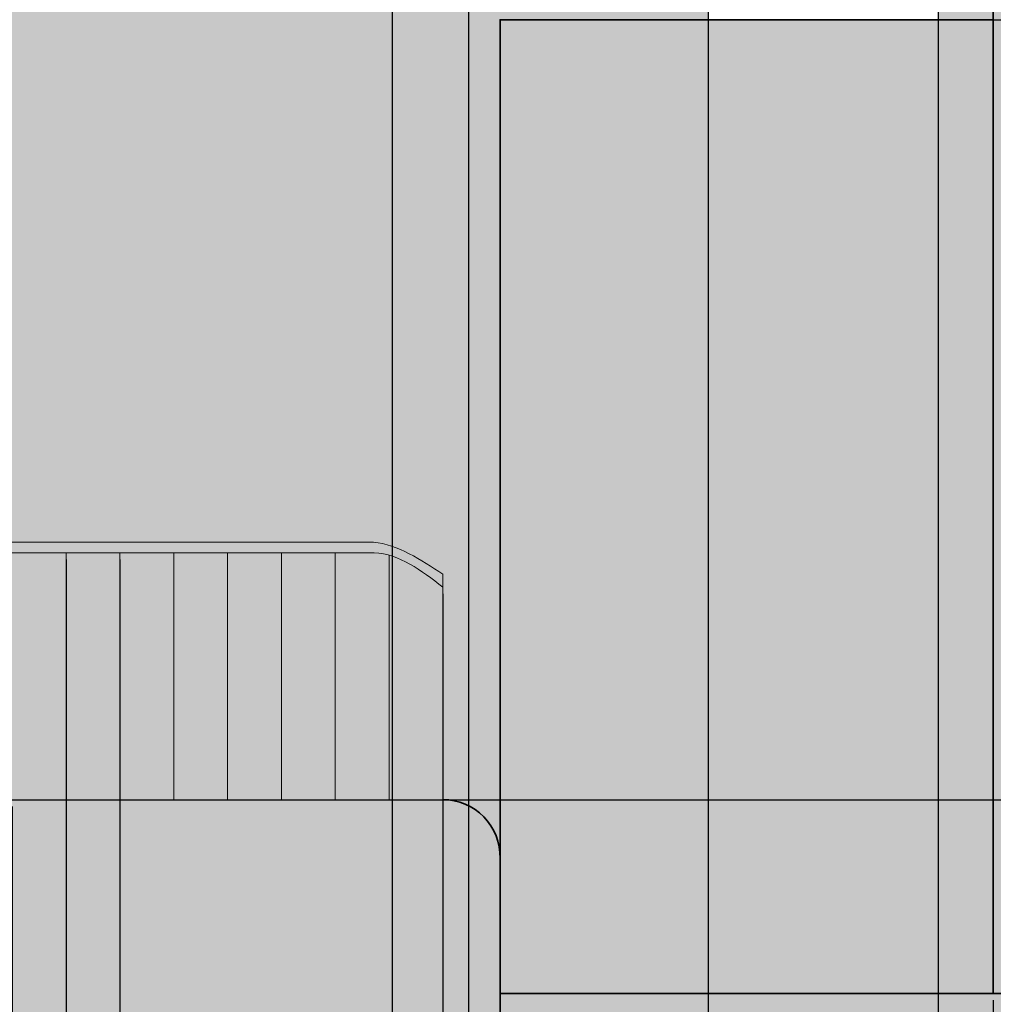
# Model space of a CAD drawing. Units: inches. Extents: x 18 to 59.8, y 2.7 to 81.2.
# Tile 6 of 9: x 44.4 to 53.4, y 29.5 to 38.7. Entities that reach past the tile are written whole.
import ezdxf

# ---------------------------------------------------------------- set-up
doc = ezdxf.new("R2010")
doc.units = ezdxf.units.IN
doc.header["$MEASUREMENT"] = 0
for name, color, linetype, lineweight in [('A-ANNO-DIMS', 2, 'Continuous', 18), ('A-ELEV', 7, 'Continuous', 35), ('A-ELEV-PATT', 8, 'Continuous', 13), ('A-ELEV-RAIL', 7, 'Continuous', 18)]:
    doc.layers.add(name, color=color, linetype=linetype, lineweight=lineweight)
doc.styles.get("Standard").update_dxf_attribs({"font": 'arial.ttf'})
doc.dimstyles.get("Standard").update_dxf_attribs({"dimtxt": 0.18, "dimasz": 0.18, "dimexe": 0.18, "dimexo": 0.0625, "dimgap": 0.09, "dimtad": 0, "dimtih": 1, "dimtoh": 1, "dimdec": 1, "dimzin": 0, "dimdsep": 46, "dimlunit": 3, "dimtxsty": 'Standard', "dimcen": 0.09, "dimadec": 0, "dimazin": 0, "dimtfac": 1, "dimtdec": 1, "dimtofl": 0, "dimtmove": 0, "dimatfit": 3, "dimfxl": 1, "dimtolj": 1, "dimtzin": 0, "dimarcsym": 0})

# ---------------------------------------------------------------- blocks, each defined once
blk = doc.blocks.new('*D23')
at = {"layer": 'A-ANNO-DIMS', "color": 0, "lineweight": -2, "transparency": 16777216}
for p, q in [((48.859971, 29.578248), (48.859971, 2.670747999999999)), ((53.440061, 29.578248), (53.440061, 2.670747999999999)), ((49.039971, 2.850747999999999), (50.82243073396998, 2.850747999999999)), ((53.260061, 2.850747999999999), (51.47760126603001, 2.850747999999999))]:
    blk.add_line(p, q, dxfattribs=at)
at = {"layer": 'A-ANNO-DIMS', "color": 0, "transparency": 16777216}
for points in [[(49.039971, 2.880747999999999), (49.039971, 2.820748), (48.859971, 2.850747999999999)], [(53.260061, 2.880747999999999), (53.260061, 2.820748), (53.440061, 2.850747999999999)]]:
    blk.add_solid(points, dxfattribs=at)
at = {"layer": 'Defpoints', "color": 0, "transparency": 16777216}
for p in [(48.859971, 29.640748), (53.440061, 29.640748), (53.440061, 2.850747999999999)]:
    blk.add_point(p, dxfattribs=at)
at = {"layer": 'A-ANNO-DIMS', "color": 0, "transparency": 16777216, "insert": (51.150016, 2.850747999999999), "char_height": 0.18, "attachment_point": 5}
blk.add_mtext('\\A1;4.58', dxfattribs=at)
blk = doc.blocks.new('*D24')
at = {"layer": 'A-ANNO-DIMS', "color": 0, "lineweight": -2, "transparency": 16777216}
for p, q in [((48.859971, 38.622063), (48.859971, 2.670748000000003)), ((50.792976, 38.622063), (50.792976, 2.670748000000003)), ((49.039971, 2.850747999999999), (49.44124157639837, 2.850747999999999)), ((50.612976, 2.850747999999999), (50.21170542360164, 2.850747999999999))]:
    blk.add_line(p, q, dxfattribs=at)
at = {"layer": 'A-ANNO-DIMS', "color": 0, "transparency": 16777216}
for points in [[(49.039971, 2.880747999999999), (49.039971, 2.820748), (48.859971, 2.850747999999999)], [(50.612976, 2.880747999999999), (50.612976, 2.820748), (50.792976, 2.850747999999999)]]:
    blk.add_solid(points, dxfattribs=at)
at = {"layer": 'Defpoints', "color": 0, "transparency": 16777216}
for p in [(48.859971, 38.684563), (50.792976, 38.684563), (50.792976, 2.850747999999999)]:
    blk.add_point(p, dxfattribs=at)
at = {"layer": 'A-ANNO-DIMS', "color": 0, "transparency": 16777216, "insert": (49.8264735, 2.850747999999999), "char_height": 0.18, "attachment_point": 5}
blk.add_mtext('\\A1;1.933', dxfattribs=at)
blk = doc.blocks.new('*D25')
at = {"layer": 'A-ANNO-DIMS', "color": 0, "lineweight": -2, "transparency": 16777216}
for p, q in [((50.792976, 41.253458), (50.792976, 2.670748000000003)), ((52.926966, 41.253458), (52.926966, 2.670748000000003)), ((50.972976, 2.850747999999999), (51.46510060436562, 2.850747999999999)), ((52.746966, 2.850747999999999), (52.25484139563437, 2.850747999999999))]:
    blk.add_line(p, q, dxfattribs=at)
at = {"layer": 'A-ANNO-DIMS', "color": 0, "transparency": 16777216}
for points in [[(50.972976, 2.880747999999999), (50.972976, 2.820748), (50.792976, 2.850747999999999)], [(52.746966, 2.880747999999999), (52.746966, 2.820748), (52.926966, 2.850747999999999)]]:
    blk.add_solid(points, dxfattribs=at)
at = {"layer": 'Defpoints', "color": 0, "transparency": 16777216}
for p in [(50.792976, 41.315958), (52.926966, 41.315958), (52.926966, 2.850747999999999)]:
    blk.add_point(p, dxfattribs=at)
at = {"layer": 'A-ANNO-DIMS', "color": 0, "transparency": 16777216, "insert": (51.859971, 2.850747999999999), "char_height": 0.18, "attachment_point": 5}
blk.add_mtext('\\A1;2.134', dxfattribs=at)
blk = doc.blocks.new('*D26')
at = {"layer": 'A-ANNO-DIMS', "color": 0, "lineweight": -2, "transparency": 16777216}
for p, q in [((52.98946600000003, 41.31595800000002), (59.62997100000006, 41.31595800000002)), ((59.44997100000005, 41.13595800000001), (59.44997100000005, 40.18222502933153)), ((59.44997100000005, 38.86456300000001), (59.44997100000005, 39.8182959706685)), ((52.98946600000003, 38.68456300000001), (59.62997100000006, 38.68456300000001))]:
    blk.add_line(p, q, dxfattribs=at)
at = {"layer": 'A-ANNO-DIMS', "color": 0, "transparency": 16777216}
for points in [[(59.41997100000005, 41.13595800000001), (59.47997100000005, 41.13595800000001), (59.44997100000005, 41.31595800000002)], [(59.41997100000005, 38.86456300000001), (59.47997100000005, 38.86456300000001), (59.44997100000005, 38.68456300000001)]]:
    blk.add_solid(points, dxfattribs=at)
at = {"layer": 'Defpoints', "color": 0, "transparency": 16777216}
for p in [(52.92696600000002, 41.31595800000002), (59.44997100000005, 41.31595800000002), (52.92696600000002, 38.68456300000001)]:
    blk.add_point(p, dxfattribs=at)
at = {"layer": 'A-ANNO-DIMS', "color": 0, "transparency": 16777216, "insert": (59.44997100000005, 40.00026049999998), "char_height": 0.18, "attachment_point": 5}
blk.add_mtext('\\A1;2.63', dxfattribs=at)
blk = doc.blocks.new('*D27')
at = {"layer": 'A-ANNO-DIMS', "color": 0, "lineweight": -2, "transparency": 16777216}
for p, q in [((30.46859000000001, 31.44074800000002), (59.62997100000006, 31.44074800000002)), ((59.44997100000005, 31.26074800000002), (59.44997100000005, 30.72265113778992)), ((59.44997100000005, 29.82074800000002), (59.44997100000005, 30.35884486221011)), ((48.92247100000003, 29.64074800000001), (59.62997100000006, 29.64074800000002))]:
    blk.add_line(p, q, dxfattribs=at)
at = {"layer": 'A-ANNO-DIMS', "color": 0, "transparency": 16777216}
for points in [[(59.41997100000005, 31.26074800000002), (59.47997100000005, 31.26074800000002), (59.44997100000005, 31.44074800000002)], [(59.41997100000005, 29.82074800000002), (59.47997100000005, 29.82074800000002), (59.44997100000005, 29.64074800000002)]]:
    blk.add_solid(points, dxfattribs=at)
at = {"layer": 'Defpoints', "color": 0, "transparency": 16777216}
for p in [(30.40609000000002, 31.44074800000002), (48.85997100000003, 29.64074800000001), (59.44997100000005, 29.64074800000002)]:
    blk.add_point(p, dxfattribs=at)
at = {"layer": 'A-ANNO-DIMS', "color": 0, "transparency": 16777216, "insert": (59.44997100000005, 30.54074799999999), "char_height": 0.18, "attachment_point": 5}
blk.add_mtext('\\A1;1.8', dxfattribs=at)
blk = doc.blocks.new('*D54')
at = {"layer": 'A-ANNO-DIMS', "color": 0, "lineweight": -2, "transparency": 16777216}
for p, q in [((28.258258, 33.771141), (28.258258, 2.670747999999999)), ((48.330239, 33.351579), (48.330239, 2.670747999999999)), ((28.438258, 2.850747999999999), (37.89900975511596, 2.850747999999999)), ((48.15023899999999, 2.850747999999999), (38.68948724488403, 2.850747999999999))]:
    blk.add_line(p, q, dxfattribs=at)
at = {"layer": 'A-ANNO-DIMS', "color": 0, "transparency": 16777216}
for points in [[(28.438258, 2.880747999999999), (28.438258, 2.820748), (28.258258, 2.850747999999999)], [(48.15023899999999, 2.880747999999999), (48.15023899999999, 2.820748), (48.330239, 2.850747999999999)]]:
    blk.add_solid(points, dxfattribs=at)
at = {"layer": 'Defpoints', "color": 0, "transparency": 16777216}
for p in [(28.258258, 33.833641), (48.330239, 33.414079), (48.330239, 2.850747999999999)]:
    blk.add_point(p, dxfattribs=at)
at = {"layer": 'A-ANNO-DIMS', "color": 0, "transparency": 16777216, "insert": (38.2942485, 2.850747999999999), "char_height": 0.18, "attachment_point": 5}
blk.add_mtext('\\A1;20.07', dxfattribs=at)
blk = doc.blocks.new('*D55')
at = {"layer": 'A-ANNO-DIMS', "color": 0, "lineweight": -2, "transparency": 16777216}
for p, q in [((44.830239, 33.671141), (44.830239, 2.670747999999999)), ((45.33023899999999, 33.671141), (45.33023899999999, 2.670747999999999)), ((44.650239, 2.850747999999999), (44.470239, 2.850747999999999)), ((45.51023899999999, 2.850747999999999), (45.690239, 2.850747999999999))]:
    blk.add_line(p, q, dxfattribs=at)
at = {"layer": 'A-ANNO-DIMS', "color": 0, "transparency": 16777216}
for points in [[(44.650239, 2.880747999999999), (44.650239, 2.820748), (44.830239, 2.850747999999999)], [(45.51023899999999, 2.880747999999999), (45.51023899999999, 2.820748), (45.33023899999999, 2.850747999999999)]]:
    blk.add_solid(points, dxfattribs=at)
at = {"layer": 'Defpoints', "color": 0, "transparency": 16777216}
for p in [(44.830239, 33.733641), (45.33023899999999, 33.733641), (45.33023899999999, 2.850747999999999)]:
    blk.add_point(p, dxfattribs=at)
at = {"layer": 'A-ANNO-DIMS', "color": 0, "transparency": 16777216, "insert": (45.94476833151432, 2.850747999999999), "char_height": 0.18, "attachment_point": 5}
blk.add_mtext('\\A1;0.5', dxfattribs=at)
blk = doc.blocks.new('*D58')
at = {"layer": 'A-ANNO-DIMS', "color": 0, "lineweight": -2, "transparency": 16777216}
for p, q in [((48.859971, 38.622063), (48.859971, 2.670748000000003)), ((44.330239, 31.378248), (44.330239, 2.670747999999999)), ((44.510239, 2.850747999999999), (46.26770390859482, 2.850747999999999)), ((48.679971, 2.850747999999999), (46.92250609140518, 2.850747999999999))]:
    blk.add_line(p, q, dxfattribs=at)
at = {"layer": 'A-ANNO-DIMS', "color": 0, "transparency": 16777216}
for points in [[(44.510239, 2.880747999999999), (44.510239, 2.820748), (44.330239, 2.850747999999999)], [(48.679971, 2.880747999999999), (48.679971, 2.820748), (48.859971, 2.850747999999999)]]:
    blk.add_solid(points, dxfattribs=at)
at = {"layer": 'Defpoints', "color": 0, "transparency": 16777216}
for p in [(48.859971, 38.684563), (44.330239, 31.440748), (48.859971, 2.850747999999999)]:
    blk.add_point(p, dxfattribs=at)
at = {"layer": 'A-ANNO-DIMS', "color": 0, "transparency": 16777216, "insert": (46.595105, 2.850747999999999), "char_height": 0.18, "attachment_point": 5}
blk.add_mtext('\\A1;4.53', dxfattribs=at)
blk = doc.blocks.new('*D61')
at = {"layer": 'A-ANNO-DIMS', "color": 0, "lineweight": -2, "transparency": 16777216}
for p, q in [((32.233824, 49.378248), (32.233824, 2.670748000000003)), ((47.859971, 49.378248), (47.859971, 2.670748000000003)), ((32.413824, 2.850747999999999), (39.59180200204638, 2.850747999999999)), ((47.679971, 2.850747999999999), (40.50199299795361, 2.850747999999999))]:
    blk.add_line(p, q, dxfattribs=at)
at = {"layer": 'A-ANNO-DIMS', "color": 0, "transparency": 16777216}
for points in [[(32.413824, 2.880747999999999), (32.413824, 2.820748), (32.233824, 2.850747999999999)], [(47.679971, 2.880747999999999), (47.679971, 2.820748), (47.859971, 2.850747999999999)]]:
    blk.add_solid(points, dxfattribs=at)
at = {"layer": 'Defpoints', "color": 0, "transparency": 16777216}
for p in [(32.233824, 49.440748), (47.859971, 49.440748), (47.859971, 2.850747999999999)]:
    blk.add_point(p, dxfattribs=at)
at = {"layer": 'A-ANNO-DIMS', "color": 0, "transparency": 16777216, "insert": (40.04689749999999, 2.850747999999999), "char_height": 0.18, "attachment_point": 5}
blk.add_mtext('\\A1;15.626', dxfattribs=at)
blk = doc.blocks.new('*D66')
at = {"layer": 'A-ANNO-DIMS', "color": 0, "lineweight": -2, "transparency": 16777216}
for p, q in [((28.803543, 51.378248), (28.803543, 2.670748000000003)), ((48.567078, 51.179103), (48.567078, 2.670748000000003)), ((28.983543, 2.850747999999999), (38.23052195975444, 2.850747999999999)), ((48.387078, 2.850747999999999), (39.14009904024556, 2.850747999999999))]:
    blk.add_line(p, q, dxfattribs=at)
at = {"layer": 'A-ANNO-DIMS', "color": 0, "transparency": 16777216}
for points in [[(28.983543, 2.880747999999999), (28.983543, 2.820748), (28.803543, 2.850747999999999)], [(48.387078, 2.880747999999999), (48.387078, 2.820748), (48.567078, 2.850747999999999)]]:
    blk.add_solid(points, dxfattribs=at)
at = {"layer": 'Defpoints', "color": 0, "transparency": 16777216}
for p in [(28.803543, 51.440748), (48.567078, 51.24160299999999), (48.567078, 2.850747999999999)]:
    blk.add_point(p, dxfattribs=at)
at = {"layer": 'A-ANNO-DIMS', "color": 0, "transparency": 16777216, "insert": (38.6853105, 2.850747999999999), "char_height": 0.18, "attachment_point": 5}
blk.add_mtext('\\A1;19.764', dxfattribs=at)

msp = doc.modelspace()

# ---------------------------------------------------------------- hatches: boundary and pattern name
at = {"layer": 'A-ELEV-PATT'}
h = msp.add_hatch(color=256, dxfattribs=at)
h.set_gradient(color1=(255, 255, 255), color2=(199, 200, 202))
h.paths.add_polyline_path([(38.85997087182833, 75.45212783007513, 0.4125526599533602), (36.85997087192615, 77.44074750583997), (21.85997087182832, 77.44074750583995), (21.85997087182832, 22.44074750583995), (22.85997087182833, 22.44074750583995), (48.85997087182833, 22.44074750583996), (48.85997087182833, 30.92342676155402, 0.4074472928332927), (48.33023903111634, 31.44074750583995), (30.40609029701442, 31.44074750583996, -0.7603989452129261), (34.01164157247843, 44.44074750583996), (47.85997087182832, 44.44074750583995, -0.4142135623730951), (48.85997087182833, 43.44074750583994), (48.85997087182833, 48.44074750583995, 0.4142135623730955), (47.85997087182832, 49.44074750583995), (32.23382408177119, 49.44074750583993, -0.2243141867862321), (27.84111392101349, 52.84266085519661, -0.8480128940945467), (38.85997087182833, 61.44074750583993)])
h.paths.add_polyline_path([(55.85997087182832, 77.44074750583995), (54.85997087182832, 77.44074750583997), (54.85997087182832, 22.24074750583996), (55.85997087182832, 22.24074750583995)])
h.paths.add_polyline_path([(54.85997087182832, 51.54074750583995), (53.44006084017791, 51.54074750583996), (53.44006084017792, 29.64074750583996), (54.85997087182832, 29.64074750583996)])
h.paths.add_polyline_path([(54.85997087182832, 61.44074750583993), (53.44006084017791, 57.44074750583993), (53.44006084017791, 51.64074750583996), (54.85997087182832, 51.64074750583996)])
h.paths.add_polyline_path([(54.85997087182832, 29.44074750583995), (54.47100875861361, 29.44074750583995), (54.47100875861361, 22.24074750583996), (54.85997087182832, 22.24074750583996)])
h.paths.add_polyline_path([(55.57447446325177, 22.24074750583995), (54.85997087182832, 22.24074750583996), (54.57447446325178, 22.24074750583996), (53.93466996146642, 21.792542566958), (54.58769880335594, 21.54947740208223)])
h.paths.add_polyline_path([(54.59913950424823, 21.54521903603421), (53.94430429933965, 21.78895655088426), (53.94430429933965, 18.44074750583995), (54.59913950424823, 18.44074750583995)])
h.paths.add_polyline_path([(53.94430429933965, 21.78895655088427), (53.93466996146642, 21.792542566958), (53.58162006229036, 21.54521903603422), (53.58162006229036, 18.44074750583995), (53.94430429933965, 18.44074750583994)])
h.paths.add_polyline_path([(53.36475139777029, 20.69276091189374), (52.89555240690669, 21.06460517556268), (52.89555240690669, 18.44074750583995), (53.3647513977703, 18.44074750583994)])
h.paths.add_polyline_path([(52.89555240690669, 21.06460517556268), (50.57752474318004, 19.44074750583995), (50.57752474318004, 18.44074750583995), (52.89555240690669, 18.44074750583995)])
h.paths.add_polyline_path([(53.58162006229036, 21.54521903603423), (52.89555240690668, 21.06460517556268), (53.3647513977703, 20.69276091189373), (53.58162006229036, 20.84468482967704)])
h.paths.add_polyline_path([(26.81093959479239, 19.44074750583995), (24.96715419074249, 20.84074750583995), (24.96715419074249, 18.44074750583995), (26.81093959479239, 18.44074750583995)])
h.paths.add_polyline_path([(24.96715419074249, 20.84074750583995), (24.41645576890079, 20.84268308307895), (24.41645576890079, 18.44074750583994), (24.96715419074249, 18.44074750583994)])
h.paths.add_polyline_path([(24.41645576890079, 20.84268308307895), (24.41645576890079, 21.25889692219009), (24.05877847081848, 21.5304839605815), (24.03006070560372, 21.51834150822755), (24.03006070560372, 18.44074750583995), (24.41645576890079, 18.44074750583995)])
h.paths.add_polyline_path([(24.03006070560372, 21.51834150822755), (23.41645576890078, 21.2588969221901), (23.41645576890078, 18.44074750583996), (24.03006070560372, 18.44074750583995)])
h.paths.add_polyline_path([(24.03006070560372, 21.51834150822755), (24.05877847081849, 21.53048396058151), (23.12336878669258, 22.24074750583995), (22.12336878669259, 22.24074750583996), (23.41645576890079, 21.2588969221901)])
h.paths.add_polyline_path([(24.41645576890079, 21.2588969221901), (24.41645576890079, 20.84268308307896), (24.96715419074249, 20.84074750583994)])
h.paths.add_polyline_path([(47.85997087182832, 18.44074750583995), (29.85997087182832, 18.44074750583995), (29.85997087182832, 6.440747505839951), (30.85997087182832, 6.440747505839937), (30.85997087182832, 17.44074750583995), (38.85997087182833, 17.44074750583995), (46.85997087182832, 17.44074750583995), (46.85997087182832, 6.440747505839937), (47.85997087182832, 6.440747505839958)])
h.paths.add_polyline_path([(54.57559250001032, 15.2149800477124), (54.57559250001032, 6.440747505839944), (55.85997087182832, 6.440747505839951), (55.85997087182832, 18.44074750583995), (47.85997087182832, 18.44074750583995), (47.85997087182832, 6.440747505839944), (49.14824210254597, 6.440747505839944), (49.14824210254597, 15.2149800477124, -1)])
h = msp.add_hatch(dxfattribs=at)
h.set_pattern_fill('ANSI31', color=256, scale=5, angle=45, style=0)
h.set_pattern_definition([(90, (0, 0), (-0.6250000000000001, 0), [])])
h.paths.add_polyline_path([(54.85997087182832, 69.44074750583995), (38.85997087182833, 69.44074750583995), (38.85997087182833, 61.44074750583995), (54.85997087182832, 61.44074750583994)])
h.paths.add_polyline_path([(54.85997087182833, 61.44074750583994), (38.85997087182833, 61.44074750583995), (36.85997087182832, 61.44074750583993, 0.4434140223301819), (27.69861713021859, 58.44074750583995), (48.85997087182833, 58.44074750583995), (48.85997087182833, 57.44074750583994), (53.44006084017792, 57.44074750583995)])
h.paths.add_polyline_path([(37.16613704638868, 59.85769359025997), (37.11866134610267, 59.85769359025997), (37.11866134610267, 59.93991004599954), (37.49943513222304, 59.93991004599954), (37.49943513222304, 59.85769359025997), (37.45195943193702, 59.85769359025997, -3.476462016968403)], flags=16)
h.paths.add_polyline_path([(42.66000754223224, 59.8390978600294), (42.61253184194623, 59.8390978600294), (42.61253184194623, 59.92131431576897), (42.9933056280666, 59.92131431576897), (42.9933056280666, 59.8390978600294), (42.94582992778058, 59.8390978600294, -3.47646201696846)], flags=16)
h.paths.add_polyline_path([(49.64399186138049, 60.00882068949565), (49.59651616109447, 60.00882068949565), (49.59651616109447, 60.09103714523522), (49.97728994721485, 60.09103714523522), (49.97728994721485, 60.00882068949565), (49.92981424692883, 60.00882068949565, -3.476462016968434)], flags=16)
h.paths.add_polyline_path([(44.46707765301489, 57.04074750583994), (32.6670776530149, 57.04074750583994), (32.6670776530149, 56.04074750583993), (44.46707765301489, 56.04074750583993)])
h.paths.add_polyline_path([(47.85997087182831, 43.44074750583994), (46.85997087182832, 43.44074750583994), (34.0116415724774, 43.44074750583994, 0.2012982920418866), (29.34810857035394, 41.44074750583995), (47.85997087182831, 41.44074750583995, 1)])
h.paths.add_polyline_path([(36.60163289663952, 42.55241488062237), (36.55415719635351, 42.55241488062236), (36.55415719635351, 42.63463133636193), (36.93493098247388, 42.63463133636193), (36.93493098247388, 42.55241488062236), (36.88745528218787, 42.55241488062236, -3.476462016968307)], flags=16)
h.paths.add_polyline_path([(42.98647563665846, 42.5780367704526), (42.93899993637245, 42.5780367704526), (42.93899993637245, 42.66025322619216), (43.31977372249282, 42.66025322619216), (43.31977372249282, 42.57803677045259), (43.2722980222068, 42.57803677045259, -3.476462016968351)], flags=16)
h.paths.add_polyline_path([(54.47100875861361, 29.44074750583995), (48.85997087182833, 29.44074750583995), (48.85997087182833, 22.24074750583995), (54.47100875861361, 22.24074750583994)])
h.paths.add_polyline_path([(54.57447446325179, 22.24074750583995), (23.12336878669258, 22.24074750583995), (26.81093959479238, 19.44074750583996), (50.57752474318005, 19.44074750583996)])
h.paths.add_polyline_path([(54.57559250001032, 15.2149800477124, 1), (49.14824210254597, 15.2149800477124), (49.14824210254597, 6.440747505839958), (54.57559250001032, 6.440747505839944)])
h.paths.add_polyline_path([(49.83226884926398, 9.122455521673542), (49.66565363924473, 9.122455521673537), (49.66565363924473, 12.60204276083839), (49.83226884926398, 12.6020427608384)], flags=16)
at = {"layer": 'A-ELEV-PATT', "transparency": 33554620}
h = msp.add_hatch(color=256, dxfattribs=at)
h.set_gradient(color1=(147, 149, 152))
edge = h.paths.add_edge_path()
edge.add_line((32.5670776530149, 55.94074750583994), (32.5670776530149, 57.14074750583994))
edge.add_line((32.5670776530149, 57.14074750583994), (44.5670776530149, 57.14074750583994))
edge.add_line((44.5670776530149, 57.14074750583994), (44.5670776530149, 55.94074750583994))
edge.add_line((44.5670776530149, 55.94074750583994), (44.56707765301487, 51.54074750583998))
edge.add_line((44.56707765301487, 51.54074750583998), (47.92075940082271, 51.54074750583998))
edge.add_spline(control_points=[(47.92075940082271, 51.54074750583998), (48.15238228194087, 51.51452682454292), (48.35972996747788, 51.37806491819363), (48.56707765301488, 51.24160301184435)], knot_values=[0, 0, 0, 0, 0.7121900809507601, 0.7121900809507601, 0.7121900809507601, 0.7121900809507601], degree=3, periodic=0)
edge.add_line((48.56707765301488, 51.24160301184435), (48.56707765301488, 49.14785428702649))
edge.add_arc((47.85997087182832, 48.44074750583995), 1, 5.739170477267294, 44.999999999999375, ccw=False)
edge.add_line((48.85495830893494, 48.54074750583996), (48.85997087182833, 48.54074750583996))
edge.add_line((48.85997087182833, 48.54074750583996), (48.85997087182833, 49.44074750583995))
edge.add_line((48.85997087182833, 49.44074750583995), (48.85997087182833, 58.44074750583995))
edge.add_line((48.85997087182833, 58.44074750583995), (27.6986171302186, 58.44074750583995))
edge.add_arc((33.63815495998532, 55.79107886226907), 6.503756879831279, 155.9580213816849, 220.80747886606)
edge.add_line((28.71539791616241, 51.54074750583994), (32.5670776530149, 51.54074750583994))
edge.add_line((32.5670776530149, 51.54074750583994), (32.5670776530149, 55.94074750583994))
edge = h.paths.add_edge_path()
edge.add_line((32.33023903111487, 40.44074750583996), (35.33023903111486, 40.44074750583996))
edge.add_line((35.33023903111486, 40.44074750583996), (38.33023903111485, 40.44074750583996))
edge.add_line((38.33023903111485, 40.44074750583996), (41.33023903111483, 40.44074750583996))
edge.add_line((41.33023903111483, 40.44074750583996), (44.33023903111482, 40.44074750583996))
edge.add_line((44.33023903111482, 40.44074750583996), (44.33023903111482, 33.83364072465343))
edge.add_line((44.33023903111482, 33.83364072465343), (47.68392077892264, 33.83364072465344))
edge.add_spline(control_points=[(47.68392077892267, 33.83364072465344), (47.91554366004082, 33.80742004335637), (48.12289134557783, 33.67095813700708), (48.33023903111483, 33.5344962306578)], knot_values=[0, 0, 0, 0, 0.7121900809507601, 0.7121900809507601, 0.7121900809507601, 0.7121900809507601], degree=3, periodic=0)
edge.add_line((48.33023903111483, 33.5344962306578), (48.33023903111483, 31.44074750583995))
edge.add_arc((48.3303844405005, 30.91101568508362), 0.5297318407134953, 1.3425044870115812, 90.01572747485528, ccw=False)
edge.add_line((48.85997087182833, 30.92342676155392), (48.85997087182833, 38.68456317332766))
edge.add_line((48.85997087182833, 38.68456317332766), (50.79297551695841, 38.68456317332766))
edge.add_line((50.79297551695841, 38.68456317332766), (50.79297551695841, 41.31595823441438))
edge.add_line((50.79297551695841, 41.31595823441438), (52.92696622669824, 41.31595823441438))
edge.add_line((52.92696622669824, 41.31595823441438), (52.92696622669824, 38.68456317332766))
edge.add_line((52.92696622669824, 38.68456317332766), (53.44006084017791, 38.68456317332766))
edge.add_line((53.44006084017791, 38.68456317332766), (53.44006084017791, 48.44074750583995))
edge.add_line((53.44006084017791, 48.44074750583995), (48.85997087182833, 48.44074750583995))
edge.add_line((48.85997087182833, 48.44074750583995), (48.85997087182832, 42.44074750583995))
edge.add_arc((47.85997087182831, 42.44074750583995), 1, -90, 0, ccw=False)
edge.add_line((47.85997087182831, 41.44074750583995), (29.34810857035394, 41.44074750583995))
edge.add_arc((34.06310194306089, 36.8836189221075), 6.557330511217327, 135.9754091201121, 207.7183105881144)
edge.add_line((28.25825772220566, 33.83364072465339), (32.33023903111487, 33.83364072465341))
edge.add_line((32.33023903111487, 33.83364072465341), (32.33023903111487, 40.44074750583996))
h.paths.add_polyline_path([(53.44006084017791, 57.44074750583995), (48.85997087182833, 57.44074750583994), (48.85997087182833, 51.64074750583996), (53.44006084017791, 51.64074750583996)])
h.paths.add_polyline_path([(29.56707765301488, 51.44074750583992), (28.80354322363853, 51.44074750583992, 0.040450980236505), (29.56707765301488, 50.71907894974708)], flags=17)
h.paths.add_polyline_path([(30.06707765301488, 51.44074750583992), (29.56707765301488, 51.44074750583992), (29.56707765301488, 50.71907894974708, 0.0237787432624053), (30.06707765301488, 50.35543166808938)], flags=17)
h.paths.add_polyline_path([(30.56707765301487, 51.44074750583993), (30.06707765301488, 51.44074750583992), (30.06707765301488, 50.35543166808938, 0.0223728768734236), (30.56707765301488, 50.05807461261393)], flags=17)
h.paths.add_polyline_path([(31.06707765301487, 51.44074750583993), (30.56707765301487, 51.44074750583993), (30.56707765301488, 50.05807461261393, 0.021345047641792), (31.06707765301488, 49.8171007041625)], flags=17)
h.paths.add_polyline_path([(31.56707765301487, 51.44074750583993), (31.06707765301487, 51.44074750583993), (31.06707765301488, 49.8171007041625, 0.0205857748313696), (31.56707765301488, 49.62589497689267)], flags=17)
h.paths.add_polyline_path([(32.06707765301488, 51.44074750583993), (31.56707765301487, 51.44074750583993), (31.56707765301488, 49.62589497689267, 0.0200299041308402), (32.06707765301488, 49.47993240164282)], flags=17)
h.paths.add_polyline_path([(32.5670776530149, 51.44074750583993), (32.06707765301488, 51.44074750583993), (32.06707765301488, 49.47993240164282, 0.0065845078177353), (32.23382408177119, 49.44074750583993), (32.5670776530149, 49.44074750583993)], flags=17)
h.paths.add_polyline_path([(45.06707765301486, 51.44074750583996), (44.56707765301487, 51.44074750583996), (44.56707765301487, 49.44074750583995), (45.06707765301488, 49.44074750583995)], flags=17)
h.paths.add_polyline_path([(45.56707765301488, 51.44074750583996), (45.06707765301486, 51.44074750583996), (45.06707765301488, 49.44074750583995), (45.56707765301488, 49.44074750583995)], flags=17)
h.paths.add_polyline_path([(46.06707765301488, 51.44074750583996), (45.56707765301488, 51.44074750583996), (45.56707765301488, 49.44074750583995), (46.06707765301488, 49.44074750583995)], flags=17)
h.paths.add_polyline_path([(46.56707765301487, 51.44074750583996), (46.06707765301488, 51.44074750583996), (46.06707765301488, 49.44074750583995), (46.56707765301487, 49.44074750583995)], flags=17)
h.paths.add_polyline_path([(47.06707765301487, 51.44074750583996), (46.56707765301487, 51.44074750583996), (46.56707765301487, 49.44074750583995), (47.06707765301487, 49.44074750583995)], flags=17)
h.paths.add_polyline_path([(47.56707765301487, 51.44074750583996), (47.06707765301487, 51.44074750583996), (47.06707765301487, 49.44074750583995), (47.56707765301488, 49.44074750583995)], flags=17)
edge = h.paths.add_edge_path(flags=17)
edge.add_spline(control_points=[(48.06707765301273, 51.41840713962396), (48.02172392661717, 51.43105064440995), (47.97524027779975, 51.4389035969284), (47.92733930740307, 51.44074750583996)], knot_values=[0.5701039528936005, 0.5701039528936005, 0.5701039528936005, 0.5701039528936005, 0.7151116034373463, 0.7151116034373463, 0.7151116034373463, 0.7151116034373644], degree=3, periodic=0)
edge.add_line((47.92733930740307, 51.44074750583996), (47.56707765301487, 51.44074750583996))
edge.add_line((47.56707765301487, 51.44074750583996), (47.56707765301488, 49.44074750583995))
edge.add_line((47.56707765301488, 49.44074750583995), (47.85997087182832, 49.44074750583995))
edge.add_arc((47.85997087182832, 48.44074750583995), 1, 78.04714410929728, 90, ccw=False)
edge.add_line((48.06707765301489, 49.41906584931846), (48.06707765301488, 51.41840713962341))
edge = h.paths.add_edge_path(flags=17)
edge.add_spline(control_points=[(48.56707765301488, 51.12118615879595), (48.40623273758901, 51.24494240176197), (48.24538782216315, 51.36869864472799), (48.06707765301273, 51.41840713962396)], knot_values=[0, 0, 0, 0, 0.5701039528936005, 0.5701039528936005, 0.5701039528936005, 0.5701039528936005], degree=3, periodic=0)
edge.add_line((48.06707765301488, 51.41840713962327), (48.06707765301489, 49.41906584931846))
edge.add_arc((47.85997087182832, 48.44074750583995), 1, 44.999999999999375, 78.04714410929728, ccw=False)
edge.add_line((48.56707765301488, 49.14785428702649), (48.56707765301488, 51.12118615879595))
h.paths.add_polyline_path([(49.35997087182833, 51.54074750583996), (48.85997087182833, 51.54074750583996), (48.85997087182833, 49.44074750583995), (48.85997087182833, 48.54074750583996), (49.35997087182833, 48.54074750583996)])
h.paths.add_polyline_path([(49.85997087182834, 51.54074750583996), (49.35997087182833, 51.54074750583996), (49.35997087182833, 48.54074750583996), (49.85997087182833, 48.54074750583996)])
h.paths.add_polyline_path([(50.35997087182834, 51.54074750583996), (49.85997087182834, 51.54074750583996), (49.85997087182833, 48.54074750583996), (50.35997087182833, 48.54074750583996)])
h.paths.add_polyline_path([(50.85997087182834, 51.54074750583996), (50.35997087182834, 51.54074750583996), (50.35997087182832, 48.54074750583996), (50.85997087182833, 48.54074750583996)])
h.paths.add_polyline_path([(51.35997087182833, 51.54074750583996), (50.85997087182834, 51.54074750583996), (50.85997087182833, 48.54074750583996), (51.35997087182833, 48.54074750583996)])
h.paths.add_polyline_path([(51.85997087182833, 51.54074750583996), (51.35997087182833, 51.54074750583996), (51.35997087182833, 48.54074750583995), (51.85997087182832, 48.54074750583995)])
h.paths.add_polyline_path([(52.35997087182834, 51.54074750583995), (51.85997087182833, 51.54074750583996), (51.85997087182832, 48.54074750583995), (52.35997087182834, 48.54074750583995)])
h.paths.add_polyline_path([(52.85997087182835, 51.54074750583995), (52.35997087182834, 51.54074750583995), (52.35997087182834, 48.54074750583995), (52.85997087182833, 48.54074750583995)])
h.paths.add_polyline_path([(53.35997087182834, 51.54074750583995), (52.85997087182835, 51.54074750583995), (52.85997087182833, 48.54074750583995), (53.35997087182834, 48.54074750583995)])
h.paths.add_polyline_path([(53.44006084017792, 38.68456317332766), (48.85997087182833, 38.68456317332766), (48.85997087182833, 30.92342676155392), (48.85997087182833, 29.64074750583995), (53.44006084017792, 29.64074750583994)])
h.paths.add_polyline_path([(28.83023903111483, 33.73364072465339), (28.31190895474052, 33.73364072465339, 0.0364451520675395), (28.83023903111484, 32.93194469741221)], flags=17)
h.paths.add_polyline_path([(29.33023903111483, 33.73364072465339), (28.83023903111483, 33.73364072465339), (28.83023903111484, 32.9319446974122, 0.0294200839082379), (29.33023903111484, 32.34505173740402)], flags=17)
h.paths.add_polyline_path([(29.83023903111483, 33.73364072465339), (29.33023903111483, 33.73364072465339), (29.33023903111484, 32.34505173740402, 0.0261691093073466), (29.83023903111483, 31.87548004603654)], flags=17)
h.paths.add_polyline_path([(30.33023903111483, 33.73364072465339), (29.83023903111483, 33.73364072465339), (29.83023903111483, 31.87548004603654, 0.0240262665661449), (30.33023903111483, 31.49248565404972)], flags=17)
h.paths.add_polyline_path([(30.83023903111483, 33.73364072465339), (30.33023903111483, 33.73364072465339), (30.33023903111483, 31.49248565404973, 0.0035005678246481), (30.40609029701443, 31.44074750583996), (30.83023903111484, 31.44074750583996)], flags=17)
h.paths.add_polyline_path([(31.33023903111483, 33.73364072465339), (30.83023903111483, 33.73364072465339), (30.83023903111484, 31.44074750583996), (31.33023903111483, 31.44074750583996)], flags=17)
h.paths.add_polyline_path([(31.83023903111483, 33.73364072465339), (31.33023903111483, 33.73364072465339), (31.33023903111483, 31.44074750583996), (31.83023903111483, 31.44074750583996)], flags=17)
h.paths.add_polyline_path([(32.33023903111487, 33.7336407246534), (31.83023903111483, 33.7336407246534), (31.83023903111483, 31.44074750583996), (32.33023903111487, 31.44074750583996)], flags=17)
h.paths.add_polyline_path([(44.83023903111482, 33.73364072465341), (44.33023903111482, 33.73364072465341), (44.33023903111482, 31.44074750583995), (44.83023903111483, 31.44074750583995)], flags=17)
h.paths.add_polyline_path([(45.33023903111483, 33.73364072465341), (44.83023903111482, 33.73364072465341), (44.83023903111483, 31.44074750583996), (45.33023903111483, 31.44074750583995)], flags=17)
h.paths.add_polyline_path([(45.83023903111483, 33.73364072465341), (45.33023903111483, 33.73364072465341), (45.33023903111483, 31.44074750583996), (45.83023903111483, 31.44074750583995)], flags=17)
h.paths.add_polyline_path([(46.33023903111483, 33.73364072465342), (45.83023903111483, 33.73364072465342), (45.83023903111483, 31.44074750583995), (46.33023903111482, 31.44074750583996)], flags=17)
h.paths.add_polyline_path([(46.83023903111482, 33.73364072465342), (46.33023903111483, 33.73364072465342), (46.33023903111482, 31.44074750583996), (46.83023903111482, 31.44074750583995)], flags=17)
h.paths.add_polyline_path([(47.33023903111482, 33.73364072465342), (46.83023903111482, 33.73364072465341), (46.83023903111482, 31.44074750583996), (47.33023903111484, 31.44074750583996)], flags=17)
edge = h.paths.add_edge_path(flags=16)
edge.add_spline(control_points=[(47.83023903111267, 33.71130035843739), (47.78488530471712, 33.7239438632234), (47.7384016558997, 33.73179681574185), (47.690500685503, 33.73364072465343)], knot_values=[0.5701039528936152, 0.5701039528936152, 0.5701039528936152, 0.5701039528936152, 0.7151116034373552, 0.7151116034373552, 0.7151116034373552, 0.7151116034373644], degree=3, periodic=0)
edge.add_line((47.69050068550314, 33.73364072465342), (47.33023903111482, 33.73364072465342))
edge.add_line((47.33023903111482, 33.73364072465342), (47.33023903111484, 31.44074750583995))
edge.add_line((47.33023903111484, 31.44074750583995), (47.83023903111484, 31.44074750583995))
edge.add_line((47.83023903111484, 31.44074750583995), (47.83023903111483, 33.71130035843684))
h.paths.add_polyline_path([(48.85997087182833, 38.68456317332766), (50.79297551695841, 38.68456317332766), (50.79297551695841, 41.31595823441438), (52.92696622669824, 41.31595823441438), (52.92696622669824, 38.68456317332766), (53.44006084017791, 38.68456317332766), (53.44006084017791, 48.44074750583995), (48.85997087182833, 48.44074750583995), (48.85997087182832, 42.44074750583995, -0.414213562373094), (47.85997087182831, 41.44074750583995), (29.34810857035394, 41.44074750583995, 0.3236799116418651), (28.25825772220566, 33.83364072465339), (32.33023903111487, 33.83364072465341), (32.33023903111487, 40.44074750583996), (35.33023903111486, 40.44074750583996), (38.33023903111485, 40.44074750583996), (41.33023903111483, 40.44074750583996), (44.33023903111482, 40.44074750583996), (44.33023903111482, 33.83364072465343), (28.25825772220566, 33.83364072465339, 0.0043266617348909), (28.31190895474052, 33.73364072465339), (28.83023903111483, 33.73364072465339), (29.33023903111483, 33.73364072465339), (29.83023903111483, 33.73364072465339), (30.33023903111483, 33.73364072465339), (30.83023903111483, 33.73364072465339), (31.33023903111483, 33.73364072465339), (31.83023903111483, 33.73364072465339), (32.33023903111487, 33.7336407246534), (47.33023903111482, 33.73364072465342), (47.33023903111484, 31.44074750583995), (47.83023903111484, 31.44074750583995), (48.33023903111591, 31.44074750583995, -0.4074472928335827), (48.85997087182833, 30.92342676155392)])
edge = h.paths.add_edge_path(flags=0)
edge.add_spline(control_points=[(47.83023903111267, 33.71130035843739), (47.78488530471713, 33.7239438632234), (47.73840165589972, 33.73179681574185), (47.69050068550303, 33.73364072465341)], knot_values=[0.5701039528936152, 0.5701039528936152, 0.5701039528936152, 0.5701039528936152, 0.7151116034373257, 0.7151116034373257, 0.7151116034373257, 0.7151116034373644], degree=3, periodic=0)
edge.add_line((47.69050068550293, 33.73364072465342), (47.33023903111482, 33.73364072465342))
edge.add_line((47.33023903111482, 33.73364072465342), (47.33023903111484, 31.44074750583995))
edge.add_line((47.33023903111484, 31.44074750583995), (47.83023903111484, 31.44074750583995))
edge.add_line((47.83023903111484, 31.44074750583995), (47.83023903111483, 33.71130035843687))
h = msp.add_hatch(color=256, dxfattribs=at)
h.set_gradient(color1=(147, 149, 152))
edge = h.paths.add_edge_path()
edge.add_line((44.33023903111482, 33.83364072465343), (47.68392077892268, 33.83364072465344))
edge.add_spline(control_points=[(47.68392077892267, 33.83364072465344), (47.91554366004082, 33.80742004335637), (48.12289134557783, 33.67095813700708), (48.33023903111483, 33.5344962306578)], knot_values=[0, 0, 0, 0, 0.7121900809507601, 0.7121900809507601, 0.7121900809507601, 0.7121900809507601], degree=3, periodic=0)
edge.add_line((48.33023903111483, 33.5344962306578), (48.33023903111483, 31.44074750583995))
edge.add_arc((48.3303844405005, 30.91101568508362), 0.5297318407134953, 1.3425044870177203, 90.01572747485528, ccw=False)
edge.add_line((48.85997087182833, 30.92342676155398), (48.85997087182833, 38.68456317332766))
edge.add_line((48.85997087182833, 38.68456317332766), (50.79297551695841, 38.68456317332766))
edge.add_line((50.79297551695841, 38.68456317332766), (50.79297551695841, 41.31595823441438))
edge.add_line((50.79297551695841, 41.31595823441438), (52.92696622669824, 41.31595823441438))
edge.add_line((52.92696622669824, 41.31595823441438), (52.92696622669824, 38.68456317332766))
edge.add_line((52.92696622669824, 38.68456317332766), (53.44006084017791, 38.68456317332766))
edge.add_line((53.44006084017791, 38.68456317332766), (53.44006084017791, 48.44074750583995))
edge.add_line((53.44006084017791, 48.44074750583995), (48.85997087182833, 48.44074750583995))
edge.add_line((48.85997087182833, 48.44074750583995), (48.85997087182832, 42.44074750583995))
edge.add_arc((47.85997087182831, 42.44074750583995), 1, -90, 0, ccw=False)
edge.add_line((47.85997087182831, 41.44074750583995), (29.34810857035394, 41.44074750583995))
edge.add_arc((34.06310194306089, 36.8836189221075), 6.557330511217328, 135.9754091201121, 207.7183105881144)
edge.add_line((28.25825772220566, 33.83364072465339), (32.33023903111487, 33.8336407246534))
edge.add_line((32.33023903111487, 33.8336407246534), (32.33023903111487, 40.44074750583996))
edge.add_line((32.33023903111487, 40.44074750583996), (35.33023903111486, 40.44074750583996))
edge.add_line((35.33023903111486, 40.44074750583996), (38.33023903111485, 40.44074750583996))
edge.add_line((38.33023903111485, 40.44074750583996), (41.33023903111483, 40.44074750583996))
edge.add_line((41.33023903111483, 40.44074750583996), (44.33023903111482, 40.44074750583996))
edge.add_line((44.33023903111482, 40.44074750583996), (44.33023903111482, 33.83364072465343))
at = {"layer": 'A-ELEV-PATT'}
h = msp.add_hatch(color=256, dxfattribs=at)
h.paths.add_polyline_path([(38.85997087182833, 17.44074750583995), (30.85997087182832, 17.44074750583995), (30.85997087182832, 6.440747505839954), (30.95997087182833, 6.440747505839954), (30.95997087182833, 17.34074750583995), (38.85997087182833, 17.34074750583995)])
h.paths.add_polyline_path([(46.85997087182832, 17.44074750583995), (38.85997087182833, 17.44074750583995), (38.85997087182833, 17.34074750583995), (46.75997087182832, 17.34074750583994), (46.75997087182832, 6.440747505839953), (46.85997087182832, 6.440747505839953)])
h.paths.add_polyline_path([(49.83226884926398, 12.6020427608384), (49.66565363924473, 12.6020427608384), (49.66565363924473, 9.122455521673542), (49.83226884926398, 9.122455521673542)])
h.paths.add_polyline_path([(48.85997087182833, 22.44074750583996), (21.85997087182832, 22.44074750583995), (21.85997087182832, 22.24074750583995), (48.85997087182833, 22.24074750583995)])
h.paths.add_polyline_path([(54.85997087182833, 29.64074750583995), (48.85997087182833, 29.64074750583995), (48.85997087182833, 29.44074750583995), (54.85997087182832, 29.44074750583995)])
edge = h.paths.add_edge_path()
edge.add_spline(control_points=[(48.33023903111483, 33.5344962306578), (48.12289134557783, 33.67095813700708), (47.91554366004082, 33.80742004335637), (47.68392077892267, 33.83364072465344)], knot_values=[0, 0, 0, 0, 0.7121900809507601, 0.7121900809507601, 0.7121900809507601, 0.7121900809507601], degree=3, periodic=0)
edge.add_line((47.68392077892267, 33.83364072465344), (28.25825772220566, 33.83364072465339))
edge.add_arc((34.06310194306086, 36.88361892210756), 6.557330511217329, 207.718310588115, 208.7099022277735)
edge.add_line((28.31190895474052, 33.73364072465339), (47.62375606275408, 33.73364072465342))
edge.add_spline(control_points=[(47.62375606275404, 33.73364072465342), (47.64610436199382, 33.73406508503794), (47.6684526612336, 33.73448944542246), (47.690500685503, 33.73364072465343)], knot_values=[0, 0, 0, 0, 0.0667446227489563, 0.0667446227489563, 0.0667446227489563, 0.0667446227489563], degree=3, periodic=0)
edge.add_spline(control_points=[(47.690500685503, 33.73364072465343), (47.7384016558997, 33.73179681574185), (47.78488530471712, 33.7239438632234), (47.83023903111267, 33.71130035843739)], knot_values=[0.5701039528936152, 0.5701039528936244, 0.5701039528936244, 0.5701039528936244, 0.7151116034373645, 0.7151116034373645, 0.7151116034373645, 0.7151116034373645], degree=3, periodic=0)
edge.add_spline(control_points=[(47.83023903111267, 33.71130035843739), (48.0085492002631, 33.66159186354143), (48.16939411568897, 33.53783562057542), (48.33023903111483, 33.41407937760941)], knot_values=[0, 0, 0, 0, 0.5701039528936152, 0.5701039528936152, 0.5701039528936152, 0.5701039528936152], degree=3, periodic=0)
edge.add_line((48.33023903111483, 33.41407937760941), (48.33023903111483, 33.5344962306578))
h = msp.add_hatch(color=256, dxfattribs=at)
edge = h.paths.add_edge_path()
edge.add_spline(control_points=[(48.33023903111483, 33.5344962306578), (48.12289134557783, 33.67095813700708), (47.91554366004082, 33.80742004335637), (47.68392077892267, 33.83364072465344)], knot_values=[0, 0, 0, 0, 0.7121900809507601, 0.7121900809507601, 0.7121900809507601, 0.7121900809507601], degree=3, periodic=0)
edge.add_line((47.68392077892267, 33.83364072465344), (28.25825772220566, 33.83364072465339))
edge.add_arc((34.06310194306085, 36.88361892210757), 6.55733051121733, 207.7183105881152, 208.7099022277736)
edge.add_line((28.31190895474052, 33.73364072465339), (47.62375606275404, 33.73364072465342))
edge.add_spline(control_points=[(47.62375606275404, 33.73364072465342), (47.64610436199382, 33.73406508503794), (47.6684526612336, 33.73448944542246), (47.690500685503, 33.73364072465343)], knot_values=[0, 0, 0, 0, 0.0667446227489563, 0.0667446227489563, 0.0667446227489563, 0.0667446227489563], degree=3, periodic=0)
edge.add_spline(control_points=[(47.690500685503, 33.73364072465343), (47.7384016558997, 33.73179681574185), (47.78488530471712, 33.7239438632234), (47.83023903111267, 33.71130035843739)], knot_values=[0.5701039528936152, 0.5701039528936244, 0.5701039528936244, 0.5701039528936244, 0.7151116034373645, 0.7151116034373645, 0.7151116034373645, 0.7151116034373645], degree=3, periodic=0)
edge.add_spline(control_points=[(47.83023903111267, 33.71130035843739), (48.0085492002631, 33.66159186354143), (48.16939411568897, 33.53783562057542), (48.33023903111483, 33.41407937760941)], knot_values=[0, 0, 0, 0, 0.5701039528936152, 0.5701039528936152, 0.5701039528936152, 0.5701039528936152], degree=3, periodic=0)
edge.add_line((48.33023903111483, 33.41407937760941), (48.33023903111483, 33.5344962306578))

# ---------------------------------------------------------------- linework, layer by layer
at = {"layer": 'A-ELEV'}
for p, q in [((53.44006084017791, 57.44074750583996), (53.44006084017792, 29.64074750583995)), ((48.85997087182833, 22.24074750583996), (48.85997087182833, 38.68456317332766)), ((54.85997087182832, 29.64074750583995), (48.85997087182833, 29.64074750583995))]:
    msp.add_line(p, q, dxfattribs=at)
msp.add_lwpolyline([(53.44006084017792, 38.68456317332766), (48.85997087182833, 38.68456317332766), (48.85997087182833, 29.64074750583995), (54.85997087182832, 29.64074750583995), (54.85997087182832, 38.68456317332766)], dxfattribs=at)
msp.add_arc((48.3303844405005, 30.91101568508362), 0.5297318407134953, 358.6574955129817, 90.01572747485535, dxfattribs=at)
at = {"layer": 'A-ELEV-RAIL'}
for p, q in [((47.68392077892265, 33.83364072465344), (28.25825772220566, 33.83364072465339)), ((47.69050068550299, 33.73364072465342), (28.31190895474052, 33.73364072465339)), ((44.83023903111483, 31.44074750583996), (44.83023903111482, 33.73364072465341)), ((45.33023903111483, 31.44074750583996), (45.33023903111483, 33.73364072465341)), ((45.83023903111483, 31.44074750583996), (45.83023903111483, 33.73364072465341)), ((46.33023903111482, 31.44074750583996), (46.33023903111483, 33.73364072465341)), ((46.83023903111481, 31.44074750583996), (46.83023903111482, 33.73364072465341)), ((47.33023903111484, 31.44074750583996), (47.33023903111482, 33.73364072465341)), ((47.83023903111484, 31.44074750583996), (47.83023903111483, 33.71130035844649)), ((48.33023903111483, 31.44074750583995), (48.33023903111483, 33.5344962306578)), ((48.3305298498838, 31.44074750583995), (30.40609029701441, 31.44074750583996))]:
    msp.add_line(p, q, dxfattribs=at)
msp.add_open_spline([(48.33023903111483, 33.5344962306578), (48.12289134557783, 33.67095813700708), (47.91554366004082, 33.80742004335637), (47.68392077892267, 33.83364072465344)], degree=3, dxfattribs=at)
msp.add_open_spline([(48.33023903111483, 33.41407937760941), (48.12848272896829, 33.56931339220206), (47.9078955922929, 33.73903610435184), (47.64610436199382, 33.73406508503793), (47.62375606275404, 33.73364072465342)], degree=3, knots=[0, 0, 0, 0, 0.7151116034373581, 0.7818562261863145, 0.7818562261863145, 0.7818562261863145, 0.7818562261863145], dxfattribs=at)

# ---------------------------------------------------------------- dimensions: what is measured, and where the dimension line sits
at = {"layer": 'A-ANNO-DIMS'}
for base, p1, p2, override, picture, middle in [((48.567078, 2.850747999999999), (28.803543, 51.440748), (48.567078, 51.24160299999999), {"dimdec": 3, "dimlfac": 1, "dimrnd": 0, "dimzin": 0, "dimdsep": 46, "dimlunit": 2}, '*D66', (38.6853105, 2.850747999999999)), ((47.859971, 2.850747999999999), (32.233824, 49.440748), (47.859971, 49.440748), {"dimdec": 3, "dimlfac": 1, "dimrnd": 0, "dimzin": 0, "dimdsep": 46, "dimlunit": 2}, '*D61', (40.04689749999999, 2.850747999999999)), ((52.926966, 2.850747999999999), (50.792976, 41.315958), (52.926966, 41.315958), {"dimdec": 3, "dimlfac": 1, "dimrnd": 0, "dimzin": 0, "dimdsep": 46, "dimlunit": 2}, '*D25', (51.859971, 2.850747999999999)), ((48.859971, 2.850747999999999), (44.330239, 31.440748), (48.859971, 38.684563), {"dimdec": 2, "dimlfac": 1, "dimrnd": 0, "dimzin": 0, "dimdsep": 46, "dimlunit": 2}, '*D58', (46.595105, 2.850747999999999)), ((50.792976, 2.850747999999999), (48.859971, 38.684563), (50.792976, 38.684563), {"dimdec": 3, "dimlfac": 1, "dimrnd": 0, "dimzin": 0, "dimdsep": 46, "dimlunit": 2}, '*D24', (49.8264735, 2.850747999999999)), ((48.330239, 2.850747999999999), (28.258258, 33.833641), (48.330239, 33.414079), {"dimdec": 2, "dimlfac": 1, "dimrnd": 0, "dimzin": 0, "dimdsep": 46, "dimlunit": 2}, '*D54', (38.2942485, 2.850747999999999)), ((45.33023899999999, 2.850747999999999), (44.830239, 33.733641), (45.33023899999999, 33.733641), {"dimdec": 1, "dimlfac": 1, "dimrnd": 0, "dimzin": 0, "dimdsep": 46, "dimlunit": 2}, '*D55', (45.94476833151432, 2.850747999999999)), ((53.440061, 2.850747999999999), (48.859971, 29.640748), (53.440061, 29.640748), {"dimdec": 2, "dimlfac": 1, "dimrnd": 0, "dimzin": 0, "dimdsep": 46, "dimlunit": 2}, '*D23', (51.150016, 2.850747999999999))]:
    dim = msp.add_linear_dim(base=base, p1=p1, p2=p2, dimstyle='Standard', override=override, dxfattribs=at)
    dim.commit()
    dim.dimension.update_dxf_attribs({"geometry": picture, "text_midpoint": middle})
for base, p1, p2, override, picture, middle in [((59.44997100000005, 41.31595800000002), (52.926966, 38.684563), (52.926966, 41.315958), {"dimdec": 2, "dimlfac": 1, "dimrnd": 0, "dimzin": 0, "dimdsep": 46, "dimlunit": 2}, '*D26', (59.44997100000005, 40.00026049999998)), ((59.44997100000005, 29.64074800000002), (30.40609, 31.440748), (48.859971, 29.640748), {"dimdec": 1, "dimlfac": 1, "dimrnd": 0, "dimzin": 0, "dimdsep": 46, "dimlunit": 2}, '*D27', (59.44997100000005, 30.54074799999999))]:
    dim = msp.add_linear_dim(base=base, p1=p1, p2=p2, angle=90, dimstyle='Standard', override=override, dxfattribs=at)
    dim.commit()
    dim.dimension.update_dxf_attribs({"geometry": picture, "text_midpoint": middle})

doc.saveas('drawing.dxf')
